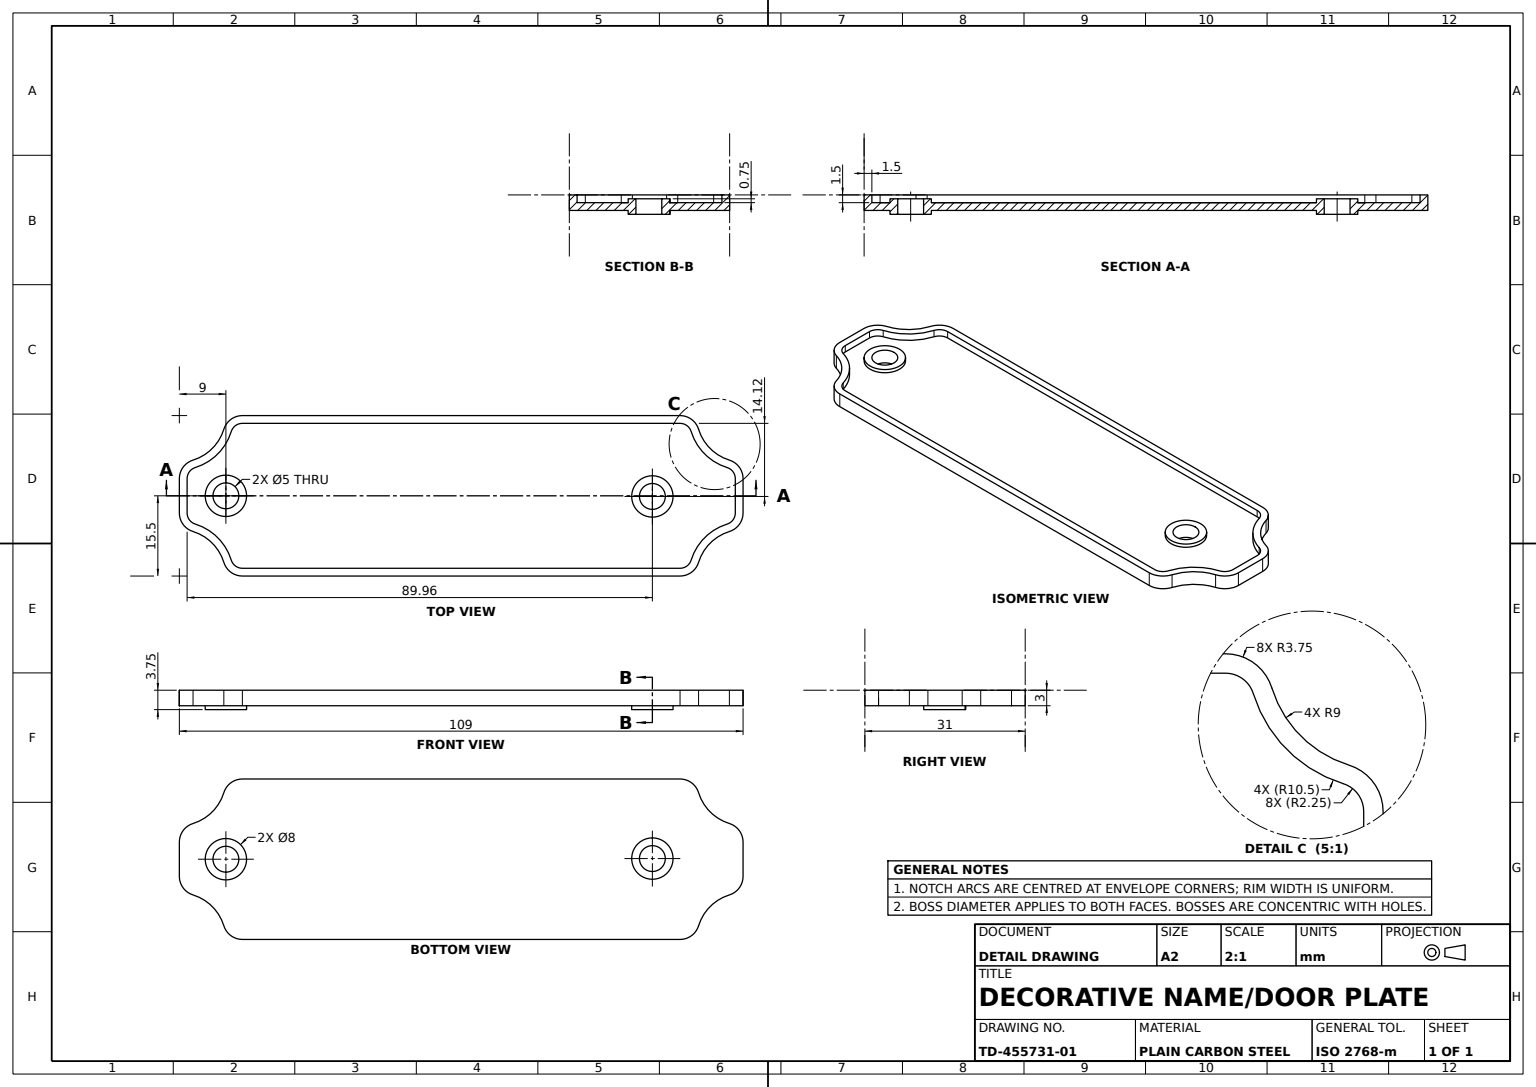
SolidWorks part; units mm, degrees
material "Plain Carbon Steel"
ref_plane "Front Plane" through (0, 0, 0) normal (0, 0, 1) x (1, 0, 0)
ref_plane "Top Plane" through (0, 0, 0) normal (0, 1, 0) x (1, 0, 0)
ref_plane "Right Plane" through (0, 0, 0) normal (1, 0, 0) x (0, 0, -1)
sketch "Plate Outline Sketch" plane through (0, 0, 0) normal (0, 1, 0) x (1, 0, 0)
  line L1 (-42.3139, 15.5) -> (42.3139, 15.5)
  line L2 (-54.5, 3.3139) -> (-54.5, -3.3139)
  line L3 (-42.3139, -15.5) -> (42.3139, -15.5)
  line L4 (54.5, 3.3139) -> (54.5, -3.3139)
  arc A0 (-51.8529, 6.8981) -> (-45.8981, 12.8529) centre (-54.5, 15.5) ccw
  arc A1 (45.8981, 12.8529) -> (51.8529, 6.8981) centre (54.5, 15.5) ccw
  arc A2 (51.8529, -6.8981) -> (45.8981, -12.8529) centre (54.5, -15.5) ccw
  arc A3 (-45.8981, -12.8529) -> (-51.8529, -6.8981) centre (-54.5, -15.5) ccw
  arc A4 (-42.3139, 15.5) -> (-45.8981, 12.8529) centre (-42.3139, 11.75) ccw
  arc A5 (45.8981, 12.8529) -> (42.3139, 15.5) centre (42.3139, 11.75) ccw
  arc A6 (42.3139, -15.5) -> (45.8981, -12.8529) centre (42.3139, -11.75) ccw
  arc A7 (-45.8981, -12.8529) -> (-42.3139, -15.5) centre (-42.3139, -11.75) ccw
  arc A12 (51.8529, -6.8981) -> (54.5, -3.3139) centre (50.75, -3.3139) ccw
  arc A13 (-51.8529, -6.8981) -> (-54.5, -3.3139) centre (-50.75, -3.3139) cw
  arc A14 (-51.8529, 6.8981) -> (-54.5, 3.3139) centre (-50.75, 3.3139) ccw
  arc A15 (51.8529, 6.8981) -> (54.5, 3.3139) centre (50.75, 3.3139) cw
  point P0 (0, 0)
  dimension "D3" = 18
  dimension "D4" = 7.5
  dimension "D5" = 3.75
  dimension "D7" = 3.75
  dimension "D1" = 31
  dimension "D2" = 54.5
  dimension "D6" = 109
  dimension "D8" = 15.5
extrude "Base Plate" add sketch "Plate Outline Sketch" along normal mid plane 3
sketch "Recess Outline Sketch" plane through (0, 1.5, 0) normal (0, 1, 0) x (1, 0, 0)
  line L8 (42.3139, 14) -> (-42.3139, 14)
  line L9 (-53, 3.3139) -> (-53, -3.3139)
  line L10 (-42.3139, -14) -> (42.3139, -14)
  line L11 (53, -3.3139) -> (53, 3.3139)
  line L12 (42.3139, 14) -> (-42.3139, 14)
  line L13 (-53, 3.3139) -> (-53, -3.3139)
  line L14 (-42.3139, -14) -> (42.3139, -14)
  line L15 (53, -3.3139) -> (53, 3.3139)
  arc A24 (44.4644, 12.4118) -> (42.3139, 14) centre (42.3139, 11.75) ccw
  arc A25 (-42.3139, 14) -> (-44.4644, 12.4118) centre (-42.3139, 11.75) ccw
  arc A26 (-51.4118, 5.4644) -> (-44.4644, 12.4118) centre (-54.5, 15.5) ccw
  arc A27 (-51.4118, 5.4644) -> (-53, 3.3139) centre (-50.75, 3.3139) ccw
  arc A28 (-53, -3.3139) -> (-51.4118, -5.4644) centre (-50.75, -3.3139) ccw
  arc A29 (-44.4644, -12.4118) -> (-51.4118, -5.4644) centre (-54.5, -15.5) ccw
  arc A30 (-44.4644, -12.4118) -> (-42.3139, -14) centre (-42.3139, -11.75) ccw
  arc A31 (42.3139, -14) -> (44.4644, -12.4118) centre (42.3139, -11.75) ccw
  arc A32 (51.4118, -5.4644) -> (44.4644, -12.4118) centre (54.5, -15.5) ccw
  arc A33 (51.4118, -5.4644) -> (53, -3.3139) centre (50.75, -3.3139) ccw
  arc A34 (53, 3.3139) -> (51.4118, 5.4644) centre (50.75, 3.3139) ccw
  arc A35 (44.4644, 12.4118) -> (51.4118, 5.4644) centre (54.5, 15.5) ccw
  arc A36 (44.4644, 12.4118) -> (42.3139, 14) centre (42.3139, 11.75) ccw
  arc A37 (-42.3139, 14) -> (-44.4644, 12.4118) centre (-42.3139, 11.75) ccw
  arc A38 (-51.4118, 5.4644) -> (-44.4644, 12.4118) centre (-54.5, 15.5) ccw
  arc A39 (-51.4118, 5.4644) -> (-53, 3.3139) centre (-50.75, 3.3139) ccw
  arc A40 (-53, -3.3139) -> (-51.4118, -5.4644) centre (-50.75, -3.3139) ccw
  arc A41 (-44.4644, -12.4118) -> (-51.4118, -5.4644) centre (-54.5, -15.5) ccw
  arc A42 (-44.4644, -12.4118) -> (-42.3139, -14) centre (-42.3139, -11.75) ccw
  arc A43 (42.3139, -14) -> (44.4644, -12.4118) centre (42.3139, -11.75) ccw
  arc A44 (51.4118, -5.4644) -> (44.4644, -12.4118) centre (54.5, -15.5) ccw
  arc A45 (51.4118, -5.4644) -> (53, -3.3139) centre (50.75, -3.3139) ccw
  arc A46 (53, 3.3139) -> (51.4118, 5.4644) centre (50.75, 3.3139) ccw
  arc A47 (44.4644, 12.4118) -> (51.4118, 5.4644) centre (54.5, 15.5) ccw
  dimension "D1" = 1.5
extrude "Top Recess 1.5mm" cut sketch "Recess Outline Sketch" against normal blind 1.5
sketch "Hole Boss Sketch" plane through (0, 0, 0) normal (0, 1, 0) x (1, 0, 0)
  line L0 (-54.5, 3.3139) -> (-54.5, -3.3139) construction
  line L1 (-53, 3.3139) -> (-53, -3.3139) construction
  line L2 (42.3139, 14) -> (-42.3139, 14) construction
  circle A0 centre (-45.5, 0) radius 2.5
  circle A1 centre (-45.5, 0) radius 4
  circle A2 centre (36.9634, -0.1232) radius 4
  circle A3 centre (36.9634, -0.1232) radius 2.5
  dimension "D1" = 8
  dimension "D2" = 5
  dimension "D3" = 8
  dimension "D4" = 9
  dimension "D5" = 89.9634
  dimension "D6" = 14.1232
extrude "Mounting Hole Bosses" add sketch "Hole Boss Sketch" along normal blind 0.75 and the other way blind 2.25
sketch "Mounting Hole Sketch" plane through (0, 0, 0) normal (0, 1, 0) x (1, 0, 0)
  circle A0 centre (-45.5, 0) radius 2.5 construction
  circle A1 centre (36.9634, -0.1232) radius 2.5
  circle A2 centre (36.9634, -0.1232) radius 2.5
  circle A3 centre (-45.5, 0) radius 2.5
  dimension "D1" = 0
extrude "Mounting Holes 2x" cut sketch "Mounting Hole Sketch" against normal blind 30.75
